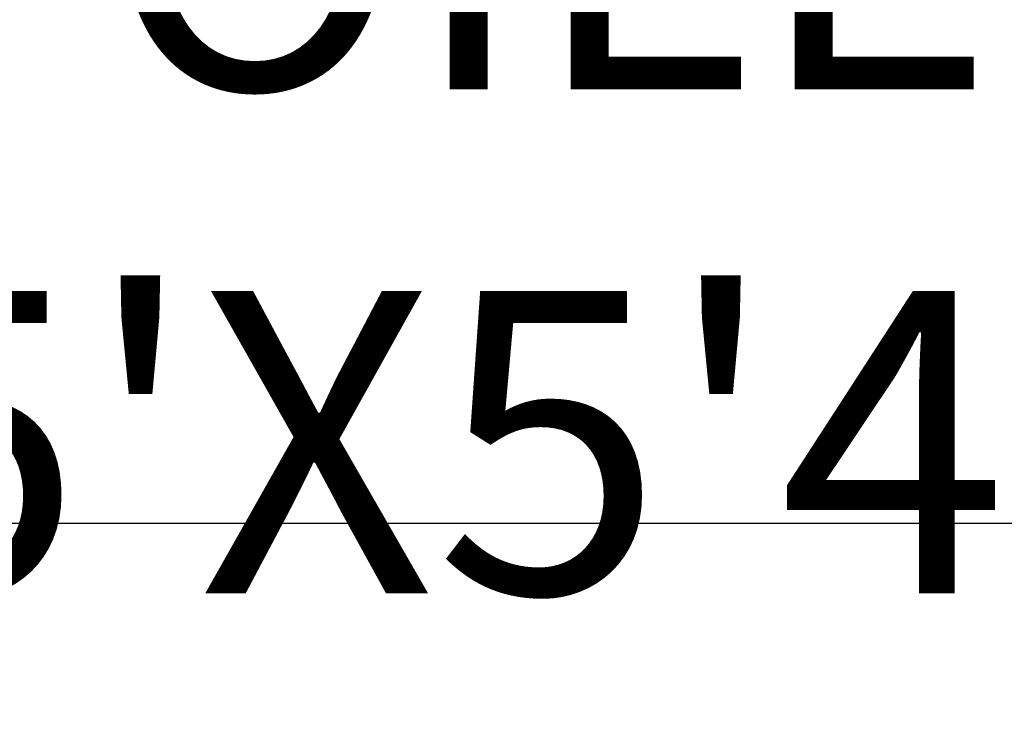
# Model space of a CAD drawing. Units: inches. Extents: x 2696 to 3240, y 1564 to 2310.
# Tile 60 of 76: x 2907 to 2936, y 2201 to 2222. Entities that reach past the tile are written whole.
import ezdxf

# ---------------------------------------------------------------- set-up
doc = ezdxf.new("R2010")
doc.units = ezdxf.units.IN
doc.layers.add('A-ANNO-DIMS', color=3, linetype='Continuous', lineweight=18)
doc.layers.add('A-AREA-IDEN', color=7, linetype='Continuous', lineweight=18)
doc.styles.add('TIMES NEW', font='times.ttf')
doc.styles.add('YQ_DIM', font='SUPEROS.SHX', dxfattribs={"width": 0.8, "bigfont": 'HZDX.SHX'})
doc.dimstyles.new('Siddhuu', dxfattribs={"dimtxt": 6, "dimasz": 2.5, "dimexe": 1.25, "dimexo": 0.625, "dimtad": 1, "dimdec": 1, "dimlunit": 4, "dimtxsty": 'TIMES NEW', "dimcen": 2.5, "dimclrd": 256, "dimclre": 1, "dimclrt": 7, "dimadec": 0, "dimazin": 0, "dimtfac": 1, "dimtdec": 1, "dimtmove": 0, "dimatfit": 3, "dimfxl": 1, "dimtolj": 1, "dimlwd": -1, "dimarcsym": 0})

# ---------------------------------------------------------------- blocks, each defined once
blk = doc.blocks.new('*D59')
at = {"layer": 'A-ANNO-DIMS', "color": 1, "lineweight": -2, "transparency": 16777216}
for p, q in [((2884.709, 1740.826), (2884.709, 2298.451)), ((2956.709, 1740.826), (2956.709, 2298.451))]:
    blk.add_line(p, q, dxfattribs=at)
at = {"layer": 'A-ANNO-DIMS', "transparency": 16777216}
blk.add_line((2887.209, 2297.201), (2954.209, 2297.201), dxfattribs=at)
for points in [[(2887.209, 2297.618), (2887.209, 2296.784), (2884.709, 2297.201)], [(2954.209, 2297.618), (2954.209, 2296.784), (2956.709, 2297.201)]]:
    blk.add_solid(points, dxfattribs=at)
at = {"layer": 'Defpoints', "color": 0, "transparency": 16777216}
for p in [(2956.709, 2297.201), (2884.709, 1740.201), (2956.709, 1740.201)]:
    blk.add_point(p, dxfattribs=at)
at = {"layer": 'A-ANNO-DIMS', "color": 7, "transparency": 16777216, "insert": (2920.709, 2300.878), "char_height": 6, "attachment_point": 5, "style": 'TIMES NEW'}
blk.add_mtext('\\A1;6\'-0"', dxfattribs=at)
blk = doc.blocks.new('*D64')
at = {"layer": 'A-ANNO-DIMS', "color": 1, "lineweight": -2, "transparency": 16777216}
for p, q in [((3073.084, 2206.701), (2709.361, 2206.701)), ((3068.584, 1989.201), (2709.361, 1989.201))]:
    blk.add_line(p, q, dxfattribs=at)
at = {"layer": 'A-ANNO-DIMS', "transparency": 16777216}
blk.add_line((2710.611, 1991.701), (2710.611, 2204.201), dxfattribs=at)
for points in [[(2710.195, 2204.201), (2711.028, 2204.201), (2710.611, 2206.701)], [(2710.195, 1991.701), (2711.028, 1991.701), (2710.611, 1989.201)]]:
    blk.add_solid(points, dxfattribs=at)
at = {"layer": 'Defpoints', "color": 0, "transparency": 16777216}
for p in [(2710.611, 2206.701), (3073.709, 2206.701), (3069.209, 1989.201)]:
    blk.add_point(p, dxfattribs=at)
at = {"layer": 'A-ANNO-DIMS', "color": 7, "transparency": 16777216, "insert": (2706.85, 2097.951), "char_height": 6, "attachment_point": 5, "rotation": 90, "style": 'TIMES NEW'}
blk.add_mtext('\\A1;18\'-1 1/2"', dxfattribs=at)

msp = doc.modelspace()

# ---------------------------------------------------------------- texts
at = {"layer": 'A-AREA-IDEN', "insert": (2902.228, 2228.623), "char_height": 9, "attachment_point": 1, "style": 'YQ_DIM'}
msp.add_mtext_dynamic_manual_height_columns('TOILET\\P5\'X5\'4.5"', width=48.00324, gutter_width=12.5, heights=[0], dxfattribs=at)

# ---------------------------------------------------------------- dimensions: what is measured, and where the dimension line sits
at = {"layer": 'A-ANNO-DIMS'}
dim = msp.add_linear_dim(base=(2956.709, 2297.201), p1=(2884.709, 1740.201), p2=(2956.709, 1740.201), dimstyle='Siddhuu', override={"dimdec": 1, "dimlfac": 1, "dimrnd": 0, "dimzin": 1, "dimdsep": 46, "dimlunit": 4, "dimfrac": 2}, dxfattribs=at)
dim.commit()
dim.dimension.update_dxf_attribs({"geometry": '*D59', "text_midpoint": (2920.709, 2300.878)})
dim = msp.add_linear_dim(base=(2710.611, 2206.701), p1=(3069.209, 1989.201), p2=(3073.709, 2206.701), angle=90, dimstyle='Siddhuu', override={"dimdec": 1, "dimlfac": 1, "dimrnd": 0, "dimzin": 1, "dimdsep": 46, "dimlunit": 4, "dimfrac": 2}, dxfattribs=at)
dim.commit()
dim.dimension.update_dxf_attribs({"geometry": '*D64', "text_midpoint": (2706.85, 2097.951)})

doc.saveas('drawing.dxf')
